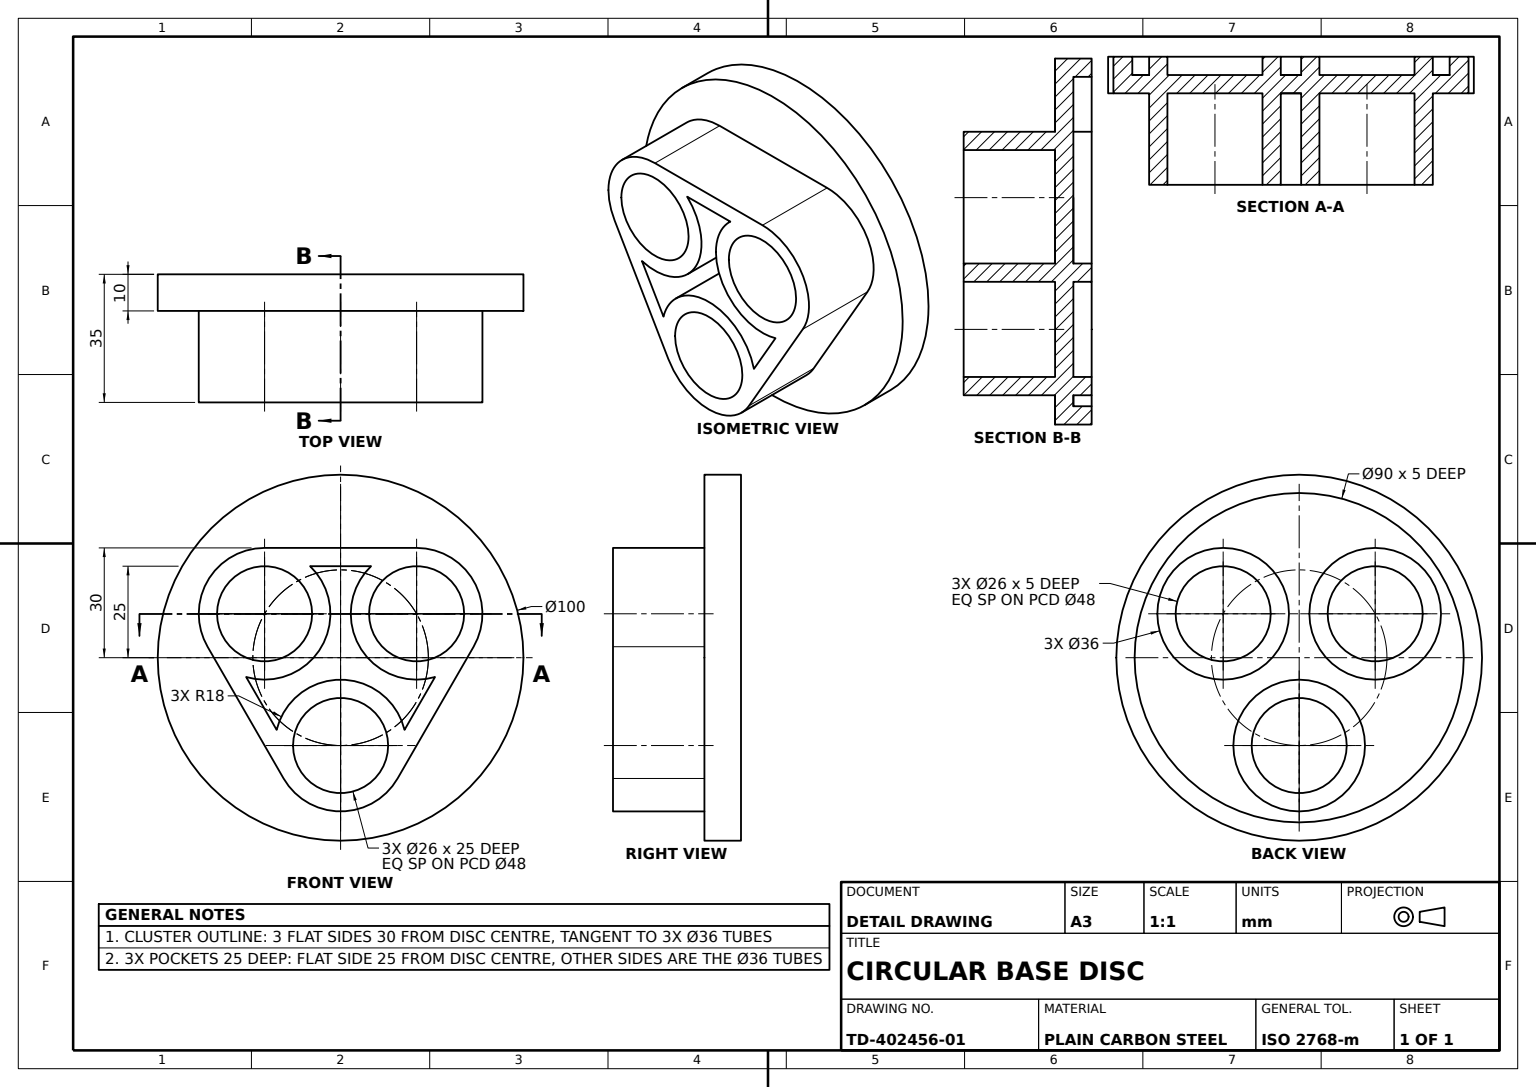
from build123d import *

# Parameters (mm, degrees)
FLANGE_PROFILE_100_R       = 50
FLANGE_100X10_DEPTH        = 10
TUBE_CLUSTER_BOSS_DEPTH    = 25
FLANGE_RECESS_PROFILE_90_R = 45
FLANGE_RECESS_90X5_DEPTH   = 5
HOLLOW_START               = -35
TUBE_PROFILES_3X_36_26_R   = 18
TUBE_PROFILES_3X_36_26_R_2 = 13
HOLLOW_TUBES_3X_36_DEPTH   = 35


with BuildPart() as part:
    # Flange Profile Ø100 → Flange Ø100x10 (new body)
    with BuildSketch(Plane.XY):
        Circle(FLANGE_PROFILE_100_R)
    extrude(amount=FLANGE_100X10_DEPTH)

    # Tube Cluster Boss Profile → Tube Cluster Boss (add)
    with BuildSketch(Plane.XY.offset(10)):
        with BuildLine():
            ThreePointArc((-8.334710093, 25), (-14.076405758, 28.703293088), (-20.784609691, 30))
            ThreePointArc((-20.784609691, 30), (-36.373066959, 21), (-36.373066959, 3))
            ThreePointArc((-36.373066959, 3), (-31.895983866, -2.161121564), (-25.817990141, -5.281929326))
            ThreePointArc((-25.817990141, -5.281929326), (-15.830471874, -5.304812004), (-7.368201826, 0))
            Line((-7.368201826, 0), (-15.784609691, 0))
            ThreePointArc((-15.784609691, 0), (-31.601263517, 19.211102551), (-7.784609691, 12))
            ThreePointArc((-7.784609691, 12), (-8.227573949, 8.635352414), (-9.526279442, 5.5))
            Line((-9.526279442, 5.5), (-5.196152423, 3))
            ThreePointArc((-5.196152423, 3), (-3.397944818, 7.341257188), (-2.784609691, 12))
            ThreePointArc((-2.784609691, 12), (-4.23018139, 19.067595321), (-8.334710093, 25))
        make_face()
        with BuildLine():
            Line((-15.784609691, 0), (-7.368201826, 0))
            ThreePointArc((-7.368201826, 0), (-6.204810298, 1.443985143), (-5.196152423, 3))
            Line((-5.196152423, 3), (-9.526279442, 5.5))
            ThreePointArc((-9.526279442, 5.5), (-12.202895082, 2.235053795), (-15.784609691, 0))
        make_face()
        with BuildLine():
            ThreePointArc((-25.817990141, -5.281929326), (-31.895983866, -2.161121564), (-36.373066959, 3))
            Line((-36.373066959, 3), (-25.980762114, -15))
            Line((-25.980762114, -15), (-21.650635095, -12.5))
            Line((-21.650635095, -12.5), (-25.817990141, -5.281929326))
        make_face()
        with BuildLine():
            Line((-21.650635095, -12.5), (-25.980762114, -15))
            Line((-25.980762114, -15), (-15.588457268, -33))
            ThreePointArc((-15.588457268, -33), (-17.819578108, -26.542171525), (-17.483280048, -19.718070674))
            Line((-17.483280048, -19.718070674), (-21.650635095, -12.5))
        make_face()
        with BuildLine():
            ThreePointArc((17.483280048, -19.718070674), (11.111374175, -9.838878436), (0, -6))
            Line((0, -6), (0, -11))
            ThreePointArc((0, -11), (9.192388155, -14.807611845), (13, -24))
            ThreePointArc((13, -24), (9.192388155, -33.192388155), (0, -37))
            Line((0, -37), (0, -42))
            ThreePointArc((0, -42), (9, -39.588457268), (15.588457268, -33))
            ThreePointArc((15.588457268, -33), (17.386664873, -28.658742812), (18, -24))
            ThreePointArc((18, -24), (17.870353114, -21.843502941), (17.483280048, -19.718070674))
        make_face()
        with BuildLine():
            Line((0, -11), (0, -6))
            ThreePointArc((0, -6), (-11.111374175, -9.838878436), (-17.483280048, -19.718070674))
            ThreePointArc((-17.483280048, -19.718070674), (-17.819578108, -26.542171525), (-15.588457268, -33))
            ThreePointArc((-15.588457268, -33), (-9, -39.588457268), (0, -42))
            Line((0, -42), (0, -37))
            ThreePointArc((0, -37), (-13, -24), (0, -11))
        make_face()
        with BuildLine():
            Line((21.650635095, -12.5), (17.483280048, -19.718070674))
            ThreePointArc((17.483280048, -19.718070674), (17.870353114, -21.843502941), (18, -24))
            ThreePointArc((18, -24), (17.386664873, -28.658742812), (15.588457268, -33))
            Line((15.588457268, -33), (25.980762114, -15))
            Line((25.980762114, -15), (21.650635095, -12.5))
        make_face()
        with BuildLine():
            Line((25.980762114, -15), (36.373066959, 3))
            ThreePointArc((36.373066959, 3), (31.895983866, -2.161121564), (25.817990141, -5.281929326))
            Line((25.817990141, -5.281929326), (21.650635095, -12.5))
            Line((21.650635095, -12.5), (25.980762114, -15))
        make_face()
        with BuildLine():
            ThreePointArc((38.784609691, 12), (33.512531752, 24.727922061), (20.784609691, 30))
            ThreePointArc((20.784609691, 30), (14.076405758, 28.703293088), (8.334710093, 25))
            ThreePointArc((8.334710093, 25), (2.965031583, 14.542171525), (5.196152423, 3))
            Line((5.196152423, 3), (9.526279442, 5.5))
            ThreePointArc((9.526279442, 5.5), (17.419962104, 24.557035742), (33.784609691, 12))
            ThreePointArc((33.784609691, 12), (27.995712242, 1.183346174), (15.784609691, 0))
            Line((15.784609691, 0), (7.368201826, 0))
            ThreePointArc((7.368201826, 0), (15.830471874, -5.304812004), (25.817990141, -5.281929326))
            ThreePointArc((25.817990141, -5.281929326), (31.895983866, -2.161121564), (36.373066959, 3))
            ThreePointArc((36.373066959, 3), (38.171274564, 7.341257188), (38.784609691, 12))
        make_face()
        with BuildLine():
            Line((9.526279442, 5.5), (5.196152423, 3))
            ThreePointArc((5.196152423, 3), (6.204810298, 1.443985143), (7.368201826, 0))
            Line((7.368201826, 0), (15.784609691, 0))
            ThreePointArc((15.784609691, 0), (12.202895082, 2.235053795), (9.526279442, 5.5))
        make_face()
        with BuildLine():
            Line((20.784609691, 30), (0, 30))
            Line((0, 30), (0, 25))
            Line((0, 25), (8.334710093, 25))
            ThreePointArc((8.334710093, 25), (14.076405758, 28.703293088), (20.784609691, 30))
        make_face()
        with BuildLine():
            Line((0, 25), (0, 30))
            Line((0, 30), (-20.784609691, 30))
            ThreePointArc((-20.784609691, 30), (-14.076405758, 28.703293088), (-8.334710093, 25))
            Line((-8.334710093, 25), (0, 25))
        make_face()
    extrude(amount=TUBE_CLUSTER_BOSS_DEPTH)

    # Flange Recess Profile Ø90 → Flange Recess Ø90x5 (cut)
    with BuildSketch(Plane(origin=(0, 0, 0), x_dir=(-1, 0, 0), z_dir=(0, 0, -1))):
        Circle(FLANGE_RECESS_PROFILE_90_R)
    extrude(amount=-FLANGE_RECESS_90X5_DEPTH, mode=Mode.SUBTRACT)

    # Tube Profiles 3xØ36-Ø26 → Hollow Tubes 3xØ36 (add)
    # profile 1 of 3: a face of its own
    with BuildSketch(Plane.XY.offset(35).offset(HOLLOW_START)):
        with Locations((20.784609691, 12)):
            Circle(TUBE_PROFILES_3X_36_26_R)
        with Locations((20.784609691, 12)):
            Circle(TUBE_PROFILES_3X_36_26_R_2, mode=Mode.SUBTRACT)
    # profile 2 of 3: a face of its own
    with BuildSketch(Plane.XY.offset(35).offset(HOLLOW_START)):
        with Locations((-20.784609691, 12)):
            Circle(TUBE_PROFILES_3X_36_26_R)
        with Locations((-20.784609691, 12)):
            Circle(TUBE_PROFILES_3X_36_26_R_2, mode=Mode.SUBTRACT)
    # profile 3 of 3: a face of its own
    with BuildSketch(Plane.XY.offset(35).offset(HOLLOW_START)):
        with Locations((0, -24)):
            Circle(TUBE_PROFILES_3X_36_26_R)
        with Locations((0, -24)):
            Circle(TUBE_PROFILES_3X_36_26_R_2, mode=Mode.SUBTRACT)
    extrude(amount=HOLLOW_TUBES_3X_36_DEPTH)


solid = part.part
